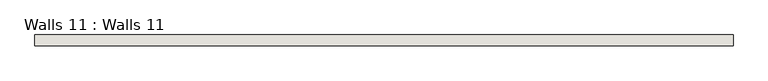
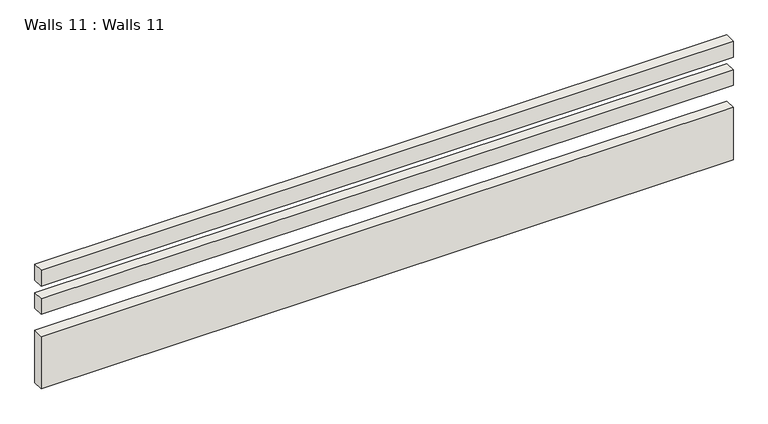
"""IFC4 building model written with IfcOpenShell, lengths in millimetres: wall geometry, Walls 11 : Walls 11."""

from ifc_helpers import new_model, si_unit, frame, origin, place, context, project, spatial, polyline, outline, extrude, source, transform, mapped, element, save


def walls_11_walls_11_77f6b4d3(model_context):
    return source(origin(), model_context, "Body", "SweptSolid", [
        extrude(outline(polyline([(-5936.6057823, -7513.1382792), (-5936.6057823, -7563.9382792), (-9197.0226654, -7563.9382792), (-9197.0226654, -7513.1382792), (-5936.6057823, -7513.1382792)])), frame((0.0, 0.0, 6096.0), z_axis=(0.0, 0.0, 1.0), x_axis=(1.0, 0.0, 0.0)), (0.0, 0.0, 1.0), 260.4628726),
        extrude(outline(polyline([(-5936.6057823, -7513.1382792), (-5936.6057823, -7563.9382792), (-9197.0226654, -7563.9382792), (-9197.0226654, -7513.1382792), (-5936.6057823, -7513.1382792)])), frame((0.0, 0.0, 6466.9720916), z_axis=(0.0, 0.0, 1.0), x_axis=(1.0, 0.0, 0.0)), (0.0, 0.0, 1.0), 77.2296068),
        extrude(outline(polyline([(-5936.6057823, -7513.1382792), (-5936.6057823, -7563.9382792), (-9197.0226654, -7563.9382792), (-9197.0226654, -7513.1382792), (-5936.6057823, -7513.1382792)])), frame((0.0, 0.0, 6607.1884053), z_axis=(0.0, 0.0, 1.0), x_axis=(1.0, 0.0, 0.0)), (0.0, 0.0, 1.0), 79.4559206),
    ])


if __name__ == "__main__":
    model = new_model("IFC4")
    model_context = context("Model", 3, world=origin())
    ifc_project = project(units=[si_unit("LENGTHUNIT", "METRE", prefix="MILLI")], contexts=[model_context])
    site = spatial("IfcSite", under=ifc_project)
    building = spatial("IfcBuilding", under=site)
    placement = place(None, origin())
    walls_11_walls_11_shape = walls_11_walls_11_77f6b4d3(model_context)
    element("IfcWall", 1, ObjectType="Walls 11 : Walls 11", at=placement, inside=building, context=model_context, shape_type="MappedRepresentation", body=[
        mapped(walls_11_walls_11_shape, transform((0.0, 0.0, 0.0), x_axis=(1.0, 0.0, 0.0), y_axis=(0.0, 1.0, 0.0), z_axis=(0.0, 0.0, 1.0))),
    ])
    save(model, "model.ifc")

# Revit data of these elements
# Element 1 (IfcWall, "Walls 11 : Walls 11")
#   Materials on its faces: "Default Wall"
# Materials
#   "Default Wall": colour RGB 80 80 80, transparency 0
